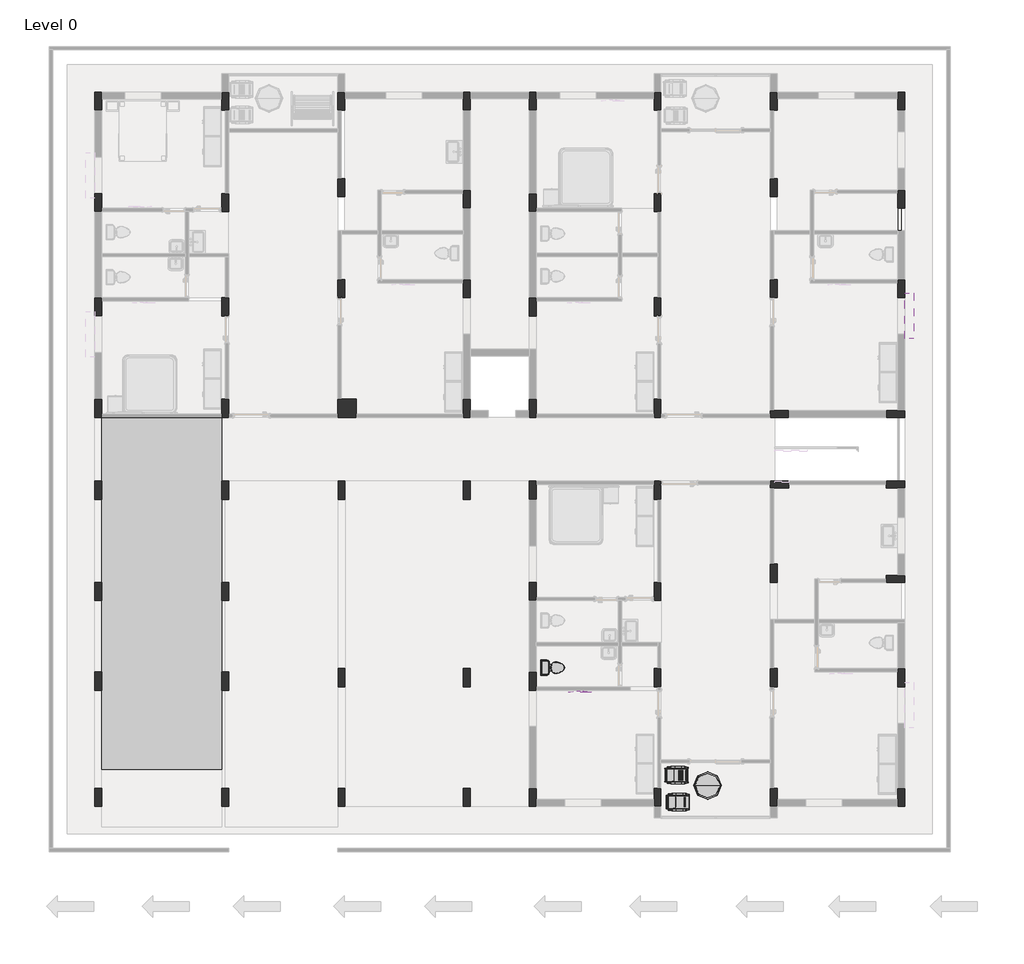
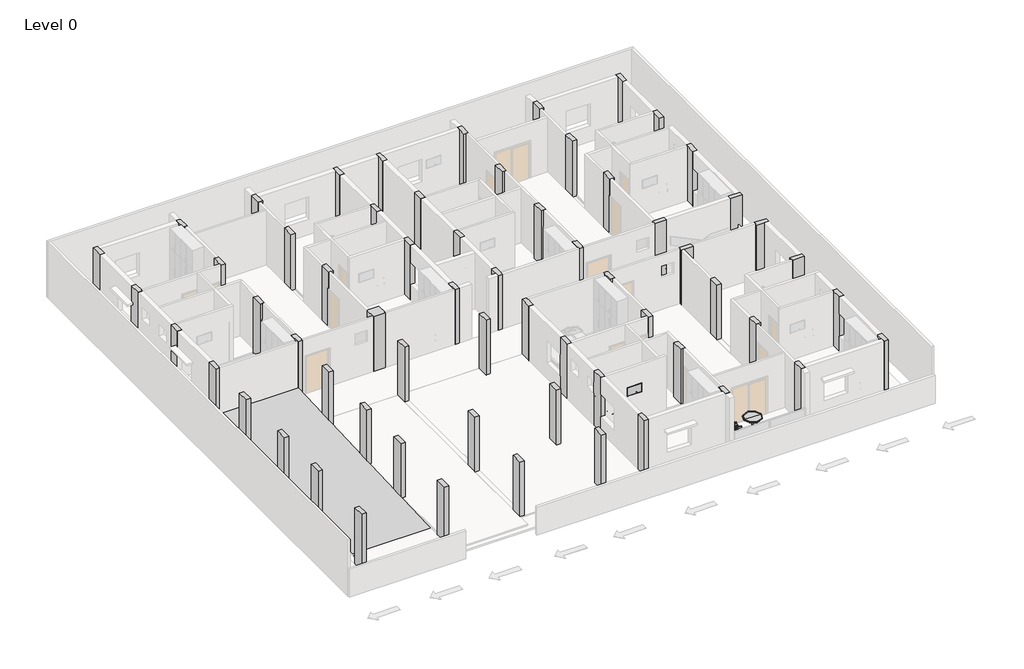
# One storey, part 5 of 6: 62 columns, 3 furniture elements, 2 slabs, 1 flow terminal, 1 proxy, 1 ramp.
"""IFC4 building model written with IfcOpenShell, lengths in millimetres."""

from ifc_helpers import new_model, si_unit, frame, origin, origin_with_axes, place, context, project, spatial, polyline, outline, extrude, faceted_brep, transform, mapped, element, save
from components import proxy_caca515e, concrete_rectangular_column_147977c2, concrete_rectangular_column_c091e905, toilet_domestic_3d_toilet_domestic_3d_ba6479b0, toilet_domestic_3d_toilet_domestic_3d_30431060, furniture_f9efd34a, adjustable_garden_chair_5339_adjustable_garden_chair_5339_e938936b, adjustable_garden_chair_5339_adjustable_garden_chair_5339_fbaf4b35, standard_832cbf63

model = new_model("IFC4")

# Units and contexts
model_context = context("Model", 3, world=origin())
ifc_project = project(units=[si_unit("LENGTHUNIT", "METRE", prefix="MILLI")], contexts=[model_context])

# Site, building, storey
site = spatial("IfcSite", under=ifc_project)
building = spatial("IfcBuilding", under=site)
storey = spatial("IfcBuildingStorey", under=building, Name="Level 0", Elevation=0.0)

# Proxy
placement = place(None, origin())
proxy_shape = proxy_caca515e(model_context)
element("IfcBuildingElementProxy", 1, Name="32\" ES6305U", ObjectType="32\" ES6305U", at=placement, inside=storey, context=model_context, shape_type="MappedRepresentation", body=[
    mapped(proxy_shape, transform((2883.4858266, -9593.9017861, 0.0), x_axis=(-1.0, 0.0, 0.0), y_axis=(0.0, -1.0, 0.0), z_axis=(0.0, 0.0, 1.0))),
])

# Columns
element("IfcColumn", 2, ObjectType="Concrete-Rectangular-Column", at=placement, inside=storey, context=model_context, shape_type="Brep", body=[
    faceted_brep([(-13249.7901539, 10361.8562752, 0.0), (-13249.7901539, 10133.2562752, 0.0), (-13249.7901539, 9752.2562752, 0.0), (-13478.3901539, 9752.2562752, 0.0), (-13478.3901539, 10361.8562752, 0.0), (-13249.7901539, 10361.8562752, 3048.0), (-13249.7901539, 10133.2562752, 3048.0), (-13249.7901539, 9752.2562752, 3048.0), (-13478.3901539, 9752.2562752, 3048.0), (-13478.3901539, 10361.8562752, 3048.0)], [[[0, 1, 2, 3, 4]], [[5, 6, 7, 2, 1, 0]], [[7, 8, 3, 2]], [[8, 9, 4, 3]], [[9, 5, 0, 4]], [[5, 9, 8, 7, 6]]]),
])
element("IfcColumn", 3, ObjectType="Concrete-Rectangular-Column", at=placement, inside=storey, context=model_context, shape_type="Brep", body=[
    faceted_brep([(-13249.7901539, 6972.1022446, 0.0), (-13249.7901539, 6362.5022446, 0.0), (-13478.3901539, 6362.5022446, 0.0), (-13478.3901539, 6972.1022446, 0.0), (-13249.7901539, 6972.1022446, 3048.0), (-13249.7901539, 6362.5022446, 3048.0), (-13249.7901539, 6972.1022446, 914.4), (-13249.7901539, 6972.1022446, 2133.6), (-13478.3901539, 6362.5022446, 3048.0), (-13478.3901539, 6972.1022446, 3048.0), (-13478.3901539, 6972.1022446, 2133.6), (-13478.3901539, 6972.1022446, 914.4)], [[[0, 1, 2, 3]], [[4, 5, 1, 0, 6, 7]], [[5, 8, 2, 1]], [[8, 9, 10, 11, 3, 2]], [[9, 4, 7, 6, 0, 3, 11, 10]], [[4, 9, 8, 5]]]),
])
element("IfcColumn", 4, ObjectType="Concrete-Rectangular-Column", at=placement, inside=storey, context=model_context, shape_type="SweptSolid", body=[
    extrude(outline(polyline([(-13249.7901539, 89.8788513), (-13249.7901539, -519.7211487), (-13478.3901539, -519.7211487), (-13478.3901539, 89.8788513), (-13249.7901539, 89.8788513)])), origin_with_axes(), (0.0, 0.0, 1.0), 3048.0),
])
element("IfcColumn", 5, ObjectType="Concrete-Rectangular-Column", at=placement, inside=storey, context=model_context, shape_type="Brep", body=[
    faceted_brep([(-9001.6401539, 10361.8562752, 0.0), (-9001.6401539, 9752.2562752, 0.0), (-9230.2401539, 9752.2562752, 0.0), (-9230.2401539, 10133.2562752, 0.0), (-9230.2401539, 10361.8562752, 0.0), (-9229.64062, 10361.8562752, 0.0), (-9001.6401539, 10361.8562752, 3048.0), (-9001.6401539, 9752.2562752, 3048.0), (-9230.2401539, 9752.2562752, 3048.0), (-9230.2401539, 10133.2562752, 3048.0), (-9230.2401539, 10361.8562752, 3048.0), (-9229.64062, 10361.8562752, 3048.0)], [[[0, 1, 2, 3, 4, 5]], [[6, 7, 1, 0]], [[7, 8, 2, 1]], [[8, 9, 10, 4, 3, 2]], [[10, 11, 6, 0, 5, 4]], [[6, 11, 10, 9, 8, 7]]]),
])
element("IfcColumn", 6, ObjectType="Concrete-Rectangular-Column", at=placement, inside=storey, context=model_context, shape_type="Brep", body=[
    faceted_brep([(-5115.4401539, 10364.1482139, 0.0), (-5115.4401539, 10363.0022446, 0.0), (-5115.4401539, 10134.4022446, 0.0), (-5115.4401539, 9754.5482139, 0.0), (-5344.0401539, 9754.5482139, 0.0), (-5344.0401539, 10364.1482139, 0.0), (-5115.4401539, 10364.1482139, 3048.0), (-5115.4401539, 10363.0022446, 3048.0), (-5115.4401539, 10134.4022446, 3048.0), (-5115.4401539, 9754.5482139, 3048.0), (-5344.0401539, 9754.5482139, 3048.0), (-5344.0401539, 10364.1482139, 3048.0)], [[[0, 1, 2, 3, 4, 5]], [[6, 7, 8, 9, 3, 2, 1, 0]], [[9, 10, 4, 3]], [[10, 11, 5, 4]], [[11, 6, 0, 5]], [[6, 11, 10, 9, 8, 7]]]),
])
element("IfcColumn", 7, ObjectType="Concrete-Rectangular-Column", at=placement, inside=storey, context=model_context, shape_type="Brep", body=[
    faceted_brep([(-924.4401539, 10363.0022446, 0.0), (-924.4401539, 10134.4022446, 0.0), (-924.4401539, 9753.4022446, 0.0), (-1153.0401539, 9753.4022446, 0.0), (-1153.0401539, 10134.4022446, 0.0), (-1153.0401539, 10363.0022446, 0.0), (-924.4401539, 10363.0022446, 3048.0), (-924.4401539, 10134.4022446, 3048.0), (-924.4401539, 9753.4022446, 3048.0), (-1153.0401539, 9753.4022446, 3048.0), (-1153.0401539, 10134.4022446, 3048.0), (-1153.0401539, 10363.0022446, 3048.0)], [[[0, 1, 2, 3, 4, 5]], [[6, 7, 8, 2, 1, 0]], [[8, 9, 3, 2]], [[9, 10, 11, 5, 4, 3]], [[11, 6, 0, 5]], [[6, 11, 10, 9, 8, 7]]]),
])
element("IfcColumn", 8, ObjectType="Concrete-Rectangular-Column", at=placement, inside=storey, context=model_context, shape_type="Brep", body=[
    faceted_brep([(1285.3598461, 10363.0022446, 0.0), (1285.3598461, 10134.4022446, 0.0), (1285.3598461, 9753.4022446, 0.0), (1056.7598461, 9753.4022446, 0.0), (1056.7598461, 10134.4022446, 0.0), (1056.7598461, 10363.0022446, 0.0), (1285.3598461, 10363.0022446, 3048.0), (1285.3598461, 10134.4022446, 3048.0), (1285.3598461, 9753.4022446, 3048.0), (1056.7598461, 9753.4022446, 3048.0), (1056.7598461, 10134.4022446, 3048.0), (1056.7598461, 10363.0022446, 3048.0)], [[[0, 1, 2, 3, 4, 5]], [[6, 7, 8, 2, 1, 0]], [[8, 9, 3, 2]], [[9, 10, 11, 5, 4, 3]], [[11, 6, 0, 5]], [[6, 11, 10, 9, 8, 7]]]),
])
element("IfcColumn", 9, ObjectType="Concrete-Rectangular-Column", at=placement, inside=storey, context=model_context, shape_type="Brep", body=[
    faceted_brep([(5457.3098461, 10364.1482139, 0.0), (5457.3098461, 9754.5482139, 0.0), (5228.7098461, 9754.5482139, 0.0), (5228.7098461, 10134.4022446, 0.0), (5228.7098461, 10363.0022446, 0.0), (5228.7098461, 10364.1482139, 0.0), (5457.3098461, 10364.1482139, 3048.0), (5457.3098461, 9754.5482139, 3048.0), (5228.7098461, 9754.5482139, 3048.0), (5228.7098461, 10134.4022446, 3048.0), (5228.7098461, 10363.0022446, 3048.0), (5228.7098461, 10364.1482139, 3048.0)], [[[0, 1, 2, 3, 4, 5]], [[6, 7, 1, 0]], [[7, 8, 2, 1]], [[8, 9, 10, 11, 5, 4, 3, 2]], [[11, 6, 0, 5]], [[6, 11, 10, 9, 8, 7]]]),
])
element("IfcColumn", 10, ObjectType="Concrete-Rectangular-Column", at=placement, inside=storey, context=model_context, shape_type="Brep", body=[
    faceted_brep([(9343.5098461, 10364.1482139, 0.0), (9343.5098461, 10135.5482139, 0.0), (9343.5098461, 9754.5482139, 0.0), (9114.9098461, 9754.5482139, 0.0), (9114.9098461, 10364.1482139, 0.0), (9343.5098461, 10364.1482139, 3048.0), (9343.5098461, 10135.5482139, 3048.0), (9343.5098461, 9754.5482139, 3048.0), (9114.9098461, 9754.5482139, 3048.0), (9114.9098461, 10364.1482139, 3048.0)], [[[0, 1, 2, 3, 4]], [[5, 6, 7, 2, 1, 0]], [[7, 8, 3, 2]], [[8, 9, 4, 3]], [[9, 5, 0, 4]], [[5, 9, 8, 7, 6]]]),
])
element("IfcColumn", 11, ObjectType="Concrete-Rectangular-Column", at=placement, inside=storey, context=model_context, shape_type="Brep", body=[
    faceted_brep([(13610.7098461, 10364.1482139, 0.0), (13610.7098461, 9754.5482139, 0.0), (13382.1098461, 9754.5482139, 0.0), (13382.1098461, 10135.5482139, 0.0), (13382.1098461, 10364.1482139, 0.0), (13610.7098461, 10364.1482139, 3048.0), (13610.7098461, 9754.5482139, 3048.0), (13382.1098461, 9754.5482139, 3048.0), (13382.1098461, 10135.5482139, 3048.0), (13382.1098461, 10364.1482139, 3048.0)], [[[0, 1, 2, 3, 4]], [[5, 6, 1, 0]], [[6, 7, 2, 1]], [[7, 8, 9, 4, 3, 2]], [[9, 5, 0, 4]], [[5, 9, 8, 7, 6]]]),
])
element("IfcColumn", 12, ObjectType="Concrete-Rectangular-Column", at=placement, inside=storey, context=model_context, shape_type="SweptSolid", body=[
    extrude(outline(polyline([(13610.7098461, 7086.4022446), (13610.7098461, 6476.8022446), (13382.1098461, 6476.8022446), (13382.1098461, 7086.4022446), (13610.7098461, 7086.4022446)])), origin_with_axes(), (0.0, 0.0, 1.0), 3048.0),
])
element("IfcColumn", 13, ObjectType="Concrete-Rectangular-Column", at=placement, inside=storey, context=model_context, shape_type="SweptSolid", body=[
    extrude(outline(polyline([(13610.7098465, 4090.3482139), (13610.7098465, 3480.7482139), (13382.1098465, 3480.7482139), (13382.1098465, 4090.3482139), (13610.7098465, 4090.3482139)])), origin_with_axes(), (0.0, 0.0, 1.0), 3048.0),
])
element("IfcColumn", 14, ObjectType="Concrete-Rectangular-Column", at=placement, inside=storey, context=model_context, shape_type="Brep", body=[
    faceted_brep([(13001.1098461, -291.1492785, 0.0), (13382.1098461, -291.1492785, 0.0), (13610.7098461, -291.1492785, 0.0), (13610.7098461, -519.7492785, 0.0), (13001.1098461, -519.7492785, 0.0), (13001.1098461, -291.1492785, 3048.0), (13382.1098461, -291.1492785, 3048.0), (13610.7098461, -291.1492785, 3048.0), (13610.7098461, -519.7492785, 3048.0), (13001.1098461, -519.7492785, 3048.0)], [[[0, 1, 2, 3, 4]], [[5, 6, 7, 2, 1, 0]], [[7, 8, 3, 2]], [[8, 9, 4, 3]], [[9, 5, 0, 4]], [[5, 9, 8, 7, 6]]]),
])
element("IfcColumn", 15, ObjectType="Concrete-Rectangular-Column", at=placement, inside=storey, context=model_context, shape_type="SweptSolid", body=[
    extrude(outline(polyline([(9116.1585903, -291.1517861), (9725.7585903, -291.1517861), (9725.7585903, -519.7517861), (9116.1585903, -519.7517861), (9116.1585903, -291.1517861)])), origin_with_axes(), (0.0, 0.0, 1.0), 3048.0),
])
element("IfcColumn", 16, ObjectType="Concrete-Rectangular-Column", at=placement, inside=storey, context=model_context, shape_type="Brep", body=[
    faceted_brep([(1056.7598461, -519.6614995, 0.0), (1056.7598461, -291.1517862, 0.0), (1056.7598461, 89.9385005, 0.0), (1285.3598461, 89.9385005, 0.0), (1285.3598461, -519.6614995, 0.0), (1056.7598461, -519.6614995, 3048.0), (1056.7598461, -291.1517862, 3048.0), (1056.7598461, 89.9385005, 3048.0), (1285.3598461, 89.9385005, 3048.0), (1285.3598461, -519.6614995, 3048.0)], [[[0, 1, 2, 3, 4]], [[5, 6, 7, 2, 1, 0]], [[7, 8, 3, 2]], [[8, 9, 4, 3]], [[9, 5, 0, 4]], [[5, 9, 8, 7, 6]]]),
])
element("IfcColumn", 17, ObjectType="Concrete-Rectangular-Column", at=placement, inside=storey, context=model_context, shape_type="Brep", body=[
    faceted_brep([(-1153.0401539, -519.7517861, 0.0), (-1153.0401539, 89.8482139, 0.0), (-924.4401539, 89.8482139, 0.0), (-924.4401539, -291.1517861, 0.0), (-924.4401539, -519.7517861, 0.0), (-1153.0401539, -519.7517861, 3048.0), (-1153.0401539, 89.8482139, 3048.0), (-924.4401539, 89.8482139, 3048.0), (-924.4401539, -291.1517861, 3048.0), (-924.4401539, -519.7517861, 3048.0)], [[[0, 1, 2, 3, 4]], [[5, 6, 1, 0]], [[6, 7, 2, 1]], [[7, 8, 9, 4, 3, 2]], [[9, 5, 0, 4]], [[5, 9, 8, 7, 6]]]),
])
element("IfcColumn", 18, ObjectType="Concrete-Rectangular-Column", at=placement, inside=storey, context=model_context, shape_type="SweptSolid", body=[
    extrude(outline(polyline([(1056.7598461, -3262.9517861), (1056.7598461, -2653.3517861), (1285.3598461, -2653.3517861), (1285.3598461, -3262.9517861), (1056.7598461, -3262.9517861)])), origin_with_axes(), (0.0, 0.0, 1.0), 3048.0),
])
element("IfcColumn", 19, ObjectType="Concrete-Rectangular-Column", at=placement, inside=storey, context=model_context, shape_type="Brep", body=[
    faceted_brep([(13610.7098461, -2881.9517861, 0.0), (13382.1098461, -2881.9517861, 0.0), (13001.1098461, -2881.9517861, 0.0), (13001.1098461, -2653.3517861, 0.0), (13610.7098461, -2653.3517861, 0.0), (13610.7098461, -2881.9517861, 3048.0), (13382.1098461, -2881.9517861, 3048.0), (13001.1098461, -2881.9517861, 3048.0), (13001.1098461, -2653.3517861, 3048.0), (13610.7098461, -2653.3517861, 3048.0)], [[[0, 1, 2, 3, 4]], [[5, 6, 7, 2, 1, 0]], [[7, 8, 3, 2]], [[8, 9, 4, 3]], [[9, 5, 0, 4]], [[5, 9, 8, 7, 6]]]),
])
element("IfcColumn", 20, ObjectType="Concrete-Rectangular-Column", at=placement, inside=storey, context=model_context, shape_type="Brep", body=[
    faceted_brep([(13610.7098461, -6044.2517861, 0.0), (13001.1098461, -6044.2517861, 0.0), (13001.1098461, -5815.6517861, 0.0), (13382.1098461, -5815.6517861, 0.0), (13610.7098461, -5815.6517861, 0.0), (13610.7098461, -6044.2517861, 3048.0), (13001.1098461, -6044.2517861, 3048.0), (13001.1098461, -5815.6517861, 3048.0), (13382.1098461, -5815.6517861, 3048.0), (13610.7098461, -5815.6517861, 3048.0)], [[[0, 1, 2, 3, 4]], [[5, 6, 1, 0]], [[6, 7, 2, 1]], [[7, 8, 9, 4, 3, 2]], [[9, 5, 0, 4]], [[5, 9, 8, 7, 6]]]),
])
element("IfcColumn", 21, ObjectType="Concrete-Rectangular-Column", at=placement, inside=storey, context=model_context, shape_type="Brep", body=[
    faceted_brep([(1285.3598461, -6044.2517861, 0.0), (1285.3598461, -6653.8517861, 0.0), (1056.7598461, -6653.8517861, 0.0), (1056.7598461, -6044.2517861, 0.0), (1285.3598461, -6044.2517861, 3048.0), (1285.3598461, -6653.8517861, 3048.0), (1285.3598461, -6044.2517861, 914.4), (1285.3598461, -6044.2517861, 2133.6), (1056.7598461, -6653.8517861, 3048.0), (1056.7598461, -6044.2517861, 3048.0), (1056.7598461, -6044.2517861, 2133.6), (1056.7598461, -6044.2517861, 914.4)], [[[0, 1, 2, 3]], [[4, 5, 1, 0, 6, 7]], [[5, 8, 2, 1]], [[8, 9, 10, 11, 3, 2]], [[9, 4, 7, 6, 0, 3, 11, 10]], [[4, 9, 8, 5]]]),
])
element("IfcColumn", 22, ObjectType="Concrete-Rectangular-Column", at=placement, inside=storey, context=model_context, shape_type="Brep", body=[
    faceted_brep([(1285.3598461, -12927.6517861, 0.0), (1285.3598461, -13308.6517861, 0.0), (1285.3598461, -13537.2517861, 0.0), (1056.7598461, -13537.2517861, 0.0), (1056.7598461, -12927.6517861, 0.0), (1285.3598461, -12927.6517861, 3048.0), (1285.3598461, -13308.6517861, 3048.0), (1285.3598461, -13537.2517861, 3048.0), (1056.7598461, -13537.2517861, 3048.0), (1056.7598461, -12927.6517861, 3048.0)], [[[0, 1, 2, 3, 4]], [[5, 6, 7, 2, 1, 0]], [[7, 8, 3, 2]], [[8, 9, 4, 3]], [[9, 5, 0, 4]], [[5, 9, 8, 7, 6]]]),
])
element("IfcColumn", 23, ObjectType="Concrete-Rectangular-Column", at=placement, inside=storey, context=model_context, shape_type="Brep", body=[
    faceted_brep([(5457.90938, -12927.6517861, 0.0), (5457.90938, -13537.2517861, 0.0), (5229.30938, -13537.2517861, 0.0), (5229.30938, -13308.6517861, 0.0), (5229.30938, -12927.6517861, 0.0), (5457.90938, -12927.6517861, 3048.0), (5457.90938, -13537.2517861, 3048.0), (5229.30938, -13537.2517861, 3048.0), (5229.30938, -13308.6517861, 3048.0), (5229.30938, -12927.6517861, 3048.0)], [[[0, 1, 2, 3, 4]], [[5, 6, 1, 0]], [[6, 7, 2, 1]], [[7, 8, 9, 4, 3, 2]], [[9, 5, 0, 4]], [[5, 9, 8, 7, 6]]]),
])
element("IfcColumn", 24, ObjectType="Concrete-Rectangular-Column", at=placement, inside=storey, context=model_context, shape_type="Brep", body=[
    faceted_brep([(9343.5098461, -12927.6517861, 0.0), (9343.5098461, -13308.6517861, 0.0), (9343.5098461, -13537.2517861, 0.0), (9114.9098461, -13537.2517861, 0.0), (9114.9098461, -12927.6517861, 0.0), (9343.5098461, -12927.6517861, 3048.0), (9343.5098461, -13308.6517861, 3048.0), (9343.5098461, -13537.2517861, 3048.0), (9114.9098461, -13537.2517861, 3048.0), (9114.9098461, -12927.6517861, 3048.0)], [[[0, 1, 2, 3, 4]], [[5, 6, 7, 2, 1, 0]], [[7, 8, 3, 2]], [[8, 9, 4, 3]], [[9, 5, 0, 4]], [[5, 9, 8, 7, 6]]]),
])
element("IfcColumn", 25, ObjectType="Concrete-Rectangular-Column", at=placement, inside=storey, context=model_context, shape_type="Brep", body=[
    faceted_brep([(13610.7098461, -12927.6517861, 0.0), (13610.7098461, -13537.2517861, 0.0), (13382.1098461, -13537.2517861, 0.0), (13382.1098461, -13308.6517861, 0.0), (13382.1098461, -12927.6517861, 0.0), (13610.7098461, -12927.6517861, 3048.0), (13610.7098461, -13537.2517861, 3048.0), (13382.1098461, -13537.2517861, 3048.0), (13382.1098461, -13308.6517861, 3048.0), (13382.1098461, -12927.6517861, 3048.0)], [[[0, 1, 2, 3, 4]], [[5, 6, 1, 0]], [[6, 7, 2, 1]], [[7, 8, 9, 4, 3, 2]], [[9, 5, 0, 4]], [[5, 9, 8, 7, 6]]]),
])
element("IfcColumn", 26, ObjectType="Concrete-Rectangular-Column", at=placement, inside=storey, context=model_context, shape_type="Brep", body=[
    faceted_brep([(13610.7098461, -8927.1824236, 0.0), (13610.7098461, -9536.7824236, 0.0), (13382.1098461, -9536.7824236, 0.0), (13382.1098461, -8927.1824236, 0.0), (13610.7098461, -8927.1824236, 3048.0), (13610.7098461, -9536.7824236, 3048.0), (13610.7098461, -9536.7824236, 2133.6), (13610.7098461, -9536.7824236, 914.4), (13382.1098461, -9536.7824236, 3048.0), (13382.1098461, -9536.7824236, 2133.6), (13382.1098461, -9536.7824236, 914.4), (13382.1098461, -8927.1824236, 3048.0)], [[[0, 1, 2, 3]], [[4, 5, 6, 7, 1, 0]], [[5, 8, 9, 10, 2, 1, 7, 6]], [[8, 11, 3, 2, 10, 9]], [[11, 4, 0, 3]], [[4, 11, 8, 5]]]),
])
element("IfcColumn", 27, ObjectType="Concrete-Rectangular-Column", at=placement, inside=storey, context=model_context, shape_type="Brep", body=[
    faceted_brep([(1285.3598461, -9041.4517861, 0.0), (1285.3598461, -9651.0517861, 0.0), (1056.7598461, -9651.0517861, 0.0), (1056.7598461, -9041.4517861, 0.0), (1285.3598461, -9041.4517861, 3048.0), (1285.3598461, -9651.0517861, 3048.0), (1285.3598461, -9651.0517861, 2133.6), (1285.3598461, -9651.0517861, 914.4), (1285.3598461, -9041.4517861, 1828.8), (1285.3598461, -9041.4517861, 2438.4), (1056.7598461, -9651.0517861, 3048.0), (1056.7598461, -9651.0517861, 2133.6), (1056.7598461, -9651.0517861, 914.4), (1056.7598461, -9041.4517861, 3048.0), (1056.7598461, -9041.4517861, 2438.4), (1056.7598461, -9041.4517861, 1828.8)], [[[0, 1, 2, 3]], [[4, 5, 6, 7, 1, 0, 8, 9]], [[5, 10, 11, 12, 2, 1, 7, 6]], [[10, 13, 14, 15, 3, 2, 12, 11]], [[13, 4, 9, 8, 0, 3, 15, 14]], [[4, 13, 10, 5]]]),
])
element("IfcColumn", 28, ObjectType="Concrete-Rectangular-Column", at=placement, inside=storey, context=model_context, shape_type="Brep", body=[
    faceted_brep([(-924.4401539, 4089.2022446, 0.0), (-924.4401539, 3479.6022446, 0.0), (-1153.0401539, 3479.6022446, 0.0), (-1153.0401539, 4089.2022446, 0.0), (-924.4401539, 4089.2022446, 3048.0), (-924.4401539, 3479.6022446, 3048.0), (-924.4401539, 3479.6022446, 2133.6), (-924.4401539, 3479.6022446, 914.4), (-1153.0401539, 3479.6022446, 3048.0), (-1153.0401539, 3479.6022446, 2133.6), (-1153.0401539, 3479.6022446, 914.4), (-1153.0401539, 4089.2022446, 3048.0)], [[[0, 1, 2, 3]], [[4, 5, 6, 7, 1, 0]], [[5, 8, 9, 10, 2, 1, 7, 6]], [[8, 11, 3, 2, 10, 9]], [[11, 4, 0, 3]], [[4, 11, 8, 5]]]),
])
element("IfcColumn", 29, ObjectType="Concrete-Rectangular-Column", at=placement, inside=storey, context=model_context, shape_type="Brep", body=[
    faceted_brep([(1285.3598461, 3481.8941832, 0.0), (1285.3598461, 2872.2941832, 0.0), (1056.7598461, 2872.2941832, 0.0), (1056.7598461, 3481.8941832, 0.0), (1285.3598461, 3481.8941832, 3048.0), (1285.3598461, 2872.2941832, 3048.0), (1285.3598461, 2872.2941832, 2133.6), (1285.3598461, 2872.2941832, 914.4), (1056.7598461, 2872.2941832, 3048.0), (1056.7598461, 2872.2941832, 2133.6), (1056.7598461, 2872.2941832, 914.4), (1056.7598461, 3481.8941832, 3048.0)], [[[0, 1, 2, 3]], [[4, 5, 6, 7, 1, 0]], [[5, 8, 9, 10, 2, 1, 7, 6]], [[8, 11, 3, 2, 10, 9]], [[11, 4, 0, 3]], [[4, 11, 8, 5]]]),
])
element("IfcColumn", 30, ObjectType="Concrete-Rectangular-Column", at=placement, inside=storey, context=model_context, shape_type="Brep", body=[
    faceted_brep([(1285.3598461, 6972.1022446, 0.0), (1285.3598461, 6477.9482139, 0.0), (1285.3598461, 6363.6482139, 0.0), (1285.3598461, 6362.5022446, 0.0), (1056.7598461, 6362.5022446, 0.0), (1056.7598461, 6972.1022446, 0.0), (1285.3598461, 6972.1022446, 3048.0), (1285.3598461, 6477.9482139, 3048.0), (1285.3598461, 6363.6482139, 3048.0), (1285.3598461, 6362.5022446, 3048.0), (1056.7598461, 6362.5022446, 3048.0), (1056.7598461, 6972.1022446, 3048.0)], [[[0, 1, 2, 3, 4, 5]], [[6, 7, 8, 9, 3, 2, 1, 0]], [[9, 10, 4, 3]], [[10, 11, 5, 4]], [[11, 6, 0, 5]], [[6, 11, 10, 9, 8, 7]]]),
])
element("IfcColumn", 31, ObjectType="Concrete-Rectangular-Column", at=placement, inside=storey, context=model_context, shape_type="SweptSolid", body=[
    extrude(outline(polyline([(-924.4401539, 7087.5482139), (-924.4401539, 6477.9482139), (-1153.0401539, 6477.9482139), (-1153.0401539, 7087.5482139), (-924.4401539, 7087.5482139)])), origin_with_axes(), (0.0, 0.0, 1.0), 3048.0),
])
element("IfcColumn", 32, ObjectType="Concrete-Rectangular-Column", at=placement, inside=storey, context=model_context, shape_type="SweptSolid", body=[
    extrude(outline(polyline([(-13249.7901539, 3480.7482139), (-13249.7901539, 2871.1482139), (-13478.3901539, 2871.1482139), (-13478.3901539, 3480.7482139), (-13249.7901539, 3480.7482139)])), origin_with_axes(), (0.0, 0.0, 1.0), 3048.0),
])
concrete_rectangular_column_shape = concrete_rectangular_column_147977c2(model_context)
element("IfcColumn", 33, ObjectType="Concrete-Rectangular-Column", at=placement, inside=storey, context=model_context, shape_type="MappedRepresentation", body=[
    mapped(concrete_rectangular_column_shape, transform((-9115.9401539, -214.9211487, 0.0), x_axis=(1.0, 0.0, 0.0), y_axis=(0.0, 1.0, 0.0), z_axis=(0.0, 0.0, 1.0))),
])
element("IfcColumn", 34, ObjectType="Concrete-Rectangular-Column", at=placement, inside=storey, context=model_context, shape_type="MappedRepresentation", body=[
    mapped(concrete_rectangular_column_shape, transform((5343.0098461, -214.8614995, 0.0), x_axis=(-1.0, 0.0, 0.0), y_axis=(0.0, -1.0, 0.0), z_axis=(0.0, 0.0, 1.0))),
])
element("IfcColumn", 35, ObjectType="Concrete-Rectangular-Column", at=placement, inside=storey, context=model_context, shape_type="MappedRepresentation", body=[
    mapped(concrete_rectangular_column_shape, transform((-5228.2486431, -2957.0057655, 0.0), x_axis=(-1.0, 0.0, 0.0), y_axis=(0.0, -1.0, 0.0), z_axis=(0.0, 0.0, 1.0))),
])
element("IfcColumn", 36, ObjectType="Concrete-Rectangular-Column", at=placement, inside=storey, context=model_context, shape_type="MappedRepresentation", body=[
    mapped(concrete_rectangular_column_shape, transform((-9115.9401539, -2958.1517861, 0.0), x_axis=(-1.0, 0.0, 0.0), y_axis=(0.0, -1.0, 0.0), z_axis=(0.0, 0.0, 1.0))),
])
element("IfcColumn", 37, ObjectType="Concrete-Rectangular-Column", at=placement, inside=storey, context=model_context, shape_type="MappedRepresentation", body=[
    mapped(concrete_rectangular_column_shape, transform((-1037.927239, -2957.0057654, 0.0), x_axis=(-1.0, 0.0, 0.0), y_axis=(0.0, -1.0, 0.0), z_axis=(0.0, 0.0, 1.0))),
])
element("IfcColumn", 38, ObjectType="Concrete-Rectangular-Column", at=placement, inside=storey, context=model_context, shape_type="MappedRepresentation", body=[
    mapped(concrete_rectangular_column_shape, transform((5343.0096341, -2958.1517861, 0.0), x_axis=(-1.0, 0.0, 0.0), y_axis=(0.0, -1.0, 0.0), z_axis=(0.0, 0.0, 1.0))),
])
element("IfcColumn", 39, ObjectType="Concrete-Rectangular-Column", at=placement, inside=storey, context=model_context, shape_type="MappedRepresentation", body=[
    mapped(concrete_rectangular_column_shape, transform((9420.9585903, -2767.6517861, 0.0), x_axis=(0.0, -1.0, 0.0), y_axis=(1.0, 0.0, 0.0), z_axis=(0.0, 0.0, 1.0))),
])
element("IfcColumn", 40, ObjectType="Concrete-Rectangular-Column", at=placement, inside=storey, context=model_context, shape_type="MappedRepresentation", body=[
    mapped(concrete_rectangular_column_shape, transform((9229.2098461, -5739.4517861, 0.0), x_axis=(1.0, 0.0, 0.0), y_axis=(0.0, 1.0, 0.0), z_axis=(0.0, 0.0, 1.0))),
])
element("IfcColumn", 41, ObjectType="Concrete-Rectangular-Column", at=placement, inside=storey, context=model_context, shape_type="MappedRepresentation", body=[
    mapped(concrete_rectangular_column_shape, transform((5343.0098461, -6349.0517861, 0.0), x_axis=(1.0, 0.0, 0.0), y_axis=(0.0, 1.0, 0.0), z_axis=(0.0, 0.0, 1.0))),
])
element("IfcColumn", 42, ObjectType="Concrete-Rectangular-Column", at=placement, inside=storey, context=model_context, shape_type="MappedRepresentation", body=[
    mapped(concrete_rectangular_column_shape, transform((-1038.0863987, -9231.9517861, 0.0), x_axis=(1.0, 0.0, 0.0), y_axis=(0.0, 1.0, 0.0), z_axis=(0.0, 0.0, 1.0))),
])
element("IfcColumn", 43, ObjectType="Concrete-Rectangular-Column", at=placement, inside=storey, context=model_context, shape_type="MappedRepresentation", body=[
    mapped(concrete_rectangular_column_shape, transform((-5228.4078028, -9231.9517861, 0.0), x_axis=(1.0, 0.0, 0.0), y_axis=(0.0, 1.0, 0.0), z_axis=(0.0, 0.0, 1.0))),
])
element("IfcColumn", 44, ObjectType="Concrete-Rectangular-Column", at=placement, inside=storey, context=model_context, shape_type="MappedRepresentation", body=[
    mapped(concrete_rectangular_column_shape, transform((-5228.4078028, -13232.4517861, 0.0), x_axis=(1.0, 0.0, 0.0), y_axis=(0.0, 1.0, 0.0), z_axis=(0.0, 0.0, 1.0))),
])
element("IfcColumn", 45, ObjectType="Concrete-Rectangular-Column", at=placement, inside=storey, context=model_context, shape_type="MappedRepresentation", body=[
    mapped(concrete_rectangular_column_shape, transform((-1038.0863987, -13232.4517861, 0.0), x_axis=(1.0, 0.0, 0.0), y_axis=(0.0, 1.0, 0.0), z_axis=(0.0, 0.0, 1.0))),
])
element("IfcColumn", 46, ObjectType="Concrete-Rectangular-Column", at=placement, inside=storey, context=model_context, shape_type="MappedRepresentation", body=[
    mapped(concrete_rectangular_column_shape, transform((-9115.9401539, -13232.4517861, 0.0), x_axis=(1.0, 0.0, 0.0), y_axis=(0.0, 1.0, 0.0), z_axis=(0.0, 0.0, 1.0))),
])
element("IfcColumn", 47, ObjectType="Concrete-Rectangular-Column", at=placement, inside=storey, context=model_context, shape_type="MappedRepresentation", body=[
    mapped(concrete_rectangular_column_shape, transform((-9115.9401539, -9346.2517861, 0.0), x_axis=(1.0, 0.0, 0.0), y_axis=(0.0, 1.0, 0.0), z_axis=(0.0, 0.0, 1.0))),
])
element("IfcColumn", 48, ObjectType="Concrete-Rectangular-Column", at=placement, inside=storey, context=model_context, shape_type="MappedRepresentation", body=[
    mapped(concrete_rectangular_column_shape, transform((-9115.9401539, -6349.0517861, 0.0), x_axis=(1.0, 0.0, 0.0), y_axis=(0.0, 1.0, 0.0), z_axis=(0.0, 0.0, 1.0))),
])
element("IfcColumn", 49, ObjectType="Concrete-Rectangular-Column", at=placement, inside=storey, context=model_context, shape_type="MappedRepresentation", body=[
    mapped(concrete_rectangular_column_shape, transform((-13363.49062, -2958.1517861, 0.0), x_axis=(1.0, 0.0, 0.0), y_axis=(0.0, 1.0, 0.0), z_axis=(0.0, 0.0, 1.0))),
])
element("IfcColumn", 50, ObjectType="Concrete-Rectangular-Column", at=placement, inside=storey, context=model_context, shape_type="MappedRepresentation", body=[
    mapped(concrete_rectangular_column_shape, transform((-13364.0901539, -6349.0517861, 0.0), x_axis=(1.0, 0.0, 0.0), y_axis=(0.0, 1.0, 0.0), z_axis=(0.0, 0.0, 1.0))),
])
element("IfcColumn", 51, ObjectType="Concrete-Rectangular-Column", at=placement, inside=storey, context=model_context, shape_type="MappedRepresentation", body=[
    mapped(concrete_rectangular_column_shape, transform((-13364.0901539, -9346.2517861, 0.0), x_axis=(1.0, 0.0, 0.0), y_axis=(0.0, 1.0, 0.0), z_axis=(0.0, 0.0, 1.0))),
])
element("IfcColumn", 52, ObjectType="Concrete-Rectangular-Column", at=placement, inside=storey, context=model_context, shape_type="MappedRepresentation", body=[
    mapped(concrete_rectangular_column_shape, transform((-13364.0901539, -13232.4517861, 0.0), x_axis=(1.0, 0.0, 0.0), y_axis=(0.0, 1.0, 0.0), z_axis=(0.0, 0.0, 1.0))),
])
element("IfcColumn", 53, ObjectType="Concrete-Rectangular-Column", at=placement, inside=storey, context=model_context, shape_type="MappedRepresentation", body=[
    mapped(concrete_rectangular_column_shape, transform((9229.2098461, -9231.9517861, 0.0), x_axis=(1.0, 0.0, 0.0), y_axis=(0.0, 1.0, 0.0), z_axis=(0.0, 0.0, 1.0))),
])
element("IfcColumn", 54, ObjectType="Concrete-Rectangular-Column", at=placement, inside=storey, context=model_context, shape_type="MappedRepresentation", body=[
    mapped(concrete_rectangular_column_shape, transform((5343.0098461, -9231.9517861, 0.0), x_axis=(1.0, 0.0, 0.0), y_axis=(0.0, 1.0, 0.0), z_axis=(0.0, 0.0, 1.0))),
])
element("IfcColumn", 55, ObjectType="Concrete-Rectangular-Column", at=placement, inside=storey, context=model_context, shape_type="MappedRepresentation", body=[
    mapped(concrete_rectangular_column_shape, transform((-9115.9401539, 3177.0941832, 0.0), x_axis=(1.0, 0.0, 0.0), y_axis=(0.0, 1.0, 0.0), z_axis=(0.0, 0.0, 1.0))),
])
element("IfcColumn", 56, ObjectType="Concrete-Rectangular-Column", at=placement, inside=storey, context=model_context, shape_type="MappedRepresentation", body=[
    mapped(concrete_rectangular_column_shape, transform((-5229.7401539, 3785.5482139, 0.0), x_axis=(1.0, 0.0, 0.0), y_axis=(0.0, 1.0, 0.0), z_axis=(0.0, 0.0, 1.0))),
])
element("IfcColumn", 57, ObjectType="Concrete-Rectangular-Column", at=placement, inside=storey, context=model_context, shape_type="MappedRepresentation", body=[
    mapped(concrete_rectangular_column_shape, transform((5343.0098461, 3177.0941832, 0.0), x_axis=(1.0, 0.0, 0.0), y_axis=(0.0, 1.0, 0.0), z_axis=(0.0, 0.0, 1.0))),
])
element("IfcColumn", 58, ObjectType="Concrete-Rectangular-Column", at=placement, inside=storey, context=model_context, shape_type="MappedRepresentation", body=[
    mapped(concrete_rectangular_column_shape, transform((-5229.7401539, 7162.6022446, 0.0), x_axis=(1.0, 0.0, 0.0), y_axis=(0.0, 1.0, 0.0), z_axis=(0.0, 0.0, 1.0))),
])
element("IfcColumn", 59, ObjectType="Concrete-Rectangular-Column", at=placement, inside=storey, context=model_context, shape_type="MappedRepresentation", body=[
    mapped(concrete_rectangular_column_shape, transform((-9115.9401539, 6667.3022446, 0.0), x_axis=(1.0, 0.0, 0.0), y_axis=(0.0, 1.0, 0.0), z_axis=(0.0, 0.0, 1.0))),
])
element("IfcColumn", 60, ObjectType="Concrete-Rectangular-Column", at=placement, inside=storey, context=model_context, shape_type="MappedRepresentation", body=[
    mapped(concrete_rectangular_column_shape, transform((5343.0098461, 6667.3022446, 0.0), x_axis=(1.0, 0.0, 0.0), y_axis=(0.0, 1.0, 0.0), z_axis=(0.0, 0.0, 1.0))),
])
element("IfcColumn", 61, ObjectType="Concrete-Rectangular-Column", at=placement, inside=storey, context=model_context, shape_type="MappedRepresentation", body=[
    mapped(concrete_rectangular_column_shape, transform((9229.2098461, 3785.5482139, 0.0), x_axis=(1.0, 0.0, 0.0), y_axis=(0.0, 1.0, 0.0), z_axis=(0.0, 0.0, 1.0))),
])
element("IfcColumn", 62, ObjectType="Concrete-Rectangular-Column", at=placement, inside=storey, context=model_context, shape_type="MappedRepresentation", body=[
    mapped(concrete_rectangular_column_shape, transform((9232.3684396, 7163.7482139, 0.0), x_axis=(1.0, 0.0, 0.0), y_axis=(0.0, 1.0, 0.0), z_axis=(0.0, 0.0, 1.0))),
])
concrete_rectangular_column_2_shape = concrete_rectangular_column_c091e905(model_context)
element("IfcColumn", 63, ObjectType="Concrete-Rectangular-Column", at=placement, inside=storey, context=model_context, shape_type="MappedRepresentation", body=[
    mapped(concrete_rectangular_column_2_shape, transform((-5039.2401539, -214.9211487, 0.0), x_axis=(1.0, 0.0, 0.0), y_axis=(0.0, 1.0, 0.0), z_axis=(0.0, 0.0, 1.0))),
])

# Flow terminal
toilet_domestic_3d_toilet_domestic_3d_shape = toilet_domestic_3d_toilet_domestic_3d_ba6479b0(model_context)
toilet_domestic_3d_toilet_domestic_3d_2_shape = toilet_domestic_3d_toilet_domestic_3d_30431060(model_context)
element("IfcFlowTerminal", 64, ObjectType="Toilet-Domestic-3D : Toilet-Domestic-3D", at=placement, inside=storey, context=model_context, shape_type="MappedRepresentation", body=[
    mapped(toilet_domestic_3d_toilet_domestic_3d_shape, transform((1932.9236467, -8898.0865272, 0.0), x_axis=(0.0, 1.0, 0.0), y_axis=(-1.0, 0.0, 0.0), z_axis=(0.0, 0.0, 1.0))),
    mapped(toilet_domestic_3d_toilet_domestic_3d_2_shape, transform((1932.9236467, -8898.0865272, 0.0), x_axis=(0.0, 1.0, 0.0), y_axis=(-1.0, 0.0, 0.0), z_axis=(0.0, 0.0, 1.0))),
])

# Furniture
furniture_shape = furniture_f9efd34a(model_context)
element("IfcFurniture", 65, ObjectType="Table-Round : 36\" Diameter", at=placement, inside=storey, context=model_context, shape_type="MappedRepresentation", body=[
    mapped(furniture_shape, transform((7019.6258765, -12843.3118957, 0.0), x_axis=(1.0, 0.0, 0.0), y_axis=(0.0, 1.0, 0.0), z_axis=(0.0, 0.0, 1.0))),
])
adjustable_garden_chair_5339_adjustable_garden_chair_5339_shape = adjustable_garden_chair_5339_adjustable_garden_chair_5339_e938936b(model_context)
element("IfcFurniture", 66, ObjectType="adjustable_garden_chair_5339 : adjustable_garden_chair_5339", at=placement, inside=storey, context=model_context, shape_type="MappedRepresentation", body=[
    mapped(adjustable_garden_chair_5339_adjustable_garden_chair_5339_shape, transform((5967.8250218, -12495.8517861, 0.0), x_axis=(0.0, 1.0, 0.0), y_axis=(-1.0, 0.0, 0.0), z_axis=(0.0, 0.0, 1.0))),
])
adjustable_garden_chair_5339_adjustable_garden_chair_5339_2_shape = adjustable_garden_chair_5339_adjustable_garden_chair_5339_fbaf4b35(model_context)
element("IfcFurniture", 67, ObjectType="adjustable_garden_chair_5339 : adjustable_garden_chair_5339", at=placement, inside=storey, context=model_context, shape_type="MappedRepresentation", body=[
    mapped(adjustable_garden_chair_5339_adjustable_garden_chair_5339_2_shape, transform((6012.6715513, -13397.191043, 0.0), x_axis=(0.0, -1.0, 0.0), y_axis=(1.0, 0.0, 0.0), z_axis=(0.0, 0.0, 1.0))),
])

# Ramp
standard_shape = standard_832cbf63(model_context)
element("IfcRamp", 68, ObjectType="Standard", at=placement, inside=storey, context=model_context, shape_type="MappedRepresentation", body=[
    mapped(standard_shape, transform((0.0, 0.0, 0.0), x_axis=(1.0, 0.0, 0.0), y_axis=(0.0, 1.0, 0.0), z_axis=(0.0, 0.0, 1.0))),
])

# Slabs
element("IfcSlab", 69, at=placement, inside=storey, context=model_context, shape_type="Brep", body=[
    faceted_brep([(10562.6567877, 5727.5022446, -50.8), (10562.6567877, 6973.2482139, -50.8), (13382.1098461, 6973.2482139, -50.8), (13382.1098461, 6476.8022446, -50.8), (13496.4098461, 6476.8022446, -50.8), (13496.4098461, 5727.5022446, -50.8), (10562.6567877, 6973.2482139, 0.0), (10562.6567877, 5727.5022446, 0.0), (13496.4098461, 5727.5022446, 0.0), (13496.4098461, 6476.8022446, 0.0), (13382.1098461, 6476.8022446, 0.0), (13382.1098461, 6973.2482139, 0.0)], [[[0, 1, 2, 3, 4, 5]], [[6, 7, 8, 9, 10, 11]], [[1, 0, 7, 6]], [[2, 1, 6, 11]], [[3, 2, 11, 10]], [[4, 3, 10, 9]], [[5, 4, 9, 8]], [[0, 5, 8, 7]]]),
    faceted_brep([(9267.64644, -521.0312258, -50.8), (9267.64644, -2653.3517861, -50.8), (1056.7598461, -2653.3517861, -50.8), (-9001.6401539, -2653.3517861, -50.8), (-9115.9401539, -2653.3517861, -50.8), (-9115.9401539, -521.0312258, -50.8), (9267.64644, -2653.3517861, 0.0), (9267.64644, -521.0312258, 0.0), (-9115.9401539, -521.0312258, 0.0), (-9115.9401539, -2653.3517861, 0.0), (-9001.6401539, -2653.3517861, 0.0), (1056.7598461, -2653.3517861, 0.0)], [[[0, 1, 2, 3, 4, 5]], [[6, 7, 8, 9, 10, 11]], [[1, 0, 7, 6]], [[1, 6, 11, 10, 9, 4, 3, 2]], [[5, 4, 9, 8]], [[0, 5, 8, 7]]]),
])
element("IfcSlab", 70, ObjectType="4\"", at=placement, inside=storey, context=model_context, shape_type="SweptSolid", body=[
    extrude(outline(polyline([(13915.5098465, 2108.5870695), (13610.7098465, 2108.5870695), (13610.7098465, 3632.5870695), (13915.5098465, 3632.5870695), (13915.5098465, 2108.5870695)])), frame((0.0, 0.0, 2108.2), z_axis=(0.0, 0.0, 1.0), x_axis=(1.0, 0.0, 0.0)), (0.0, 0.0, 1.0), 101.6),
])

save(model, "model.ifc")

# Revit data of these elements
# Type "32\" ES6305U"
#   URL = "http://www.samsung.com"
#   Model = "32ES6305U"
#   Manufacturer = "Samsung"
#   Description = "3D led smart tv, 6 series"
#   Width = 2' - 5.13386"
#   Placement height [instance default] = 5' - 6.92913"
#   Outputs inset = 0' - 0.3937"
#   Output size = 0' - 0.15748"
#   Inset corners = 0' - 0.3937"
#   Inset component exit = 0' - 1.77165"
#   Inset body = 0' - 0.7874"
#   Height = 1' - 5.6378"
#   Depth screen = 0' - 0.62992"
#   Depth frame edge = 0' - 0.03937"
#   Depth distance = 0' - 1.1811"
#   Depth body = 0' - 0.86614"
#   Screen material = TV Screen material
#   Frame material = TV Frame material
#   Body material = TV Body material
#   Default Elevation = 0
# Type "Concrete-Rectangular-Column"
#   Assembly Code = "B10"
#   b = 0' - 9"
#   h = 2' - 0"
#   Structural Material [instance default] = Concrete, Cast-in-Place gray
# Type "Concrete-Rectangular-Column"
#   Assembly Code = "B10"
#   b = 2' - 0"
#   h = 2' - 0"
#   Structural Material [instance default] = Concrete, Cast-in-Place gray
# Type "Toilet-Domestic-3D : Toilet-Domestic-3D"
#   Assembly Code = "D2010110"
#   Toilet - Bowl/Basin Material = Porcelain, Linen
#   Toilet - Seat Material = Laminate, Linen, Matte
#   Default Elevation = 0
# Type "Table-Round : 36\" Diameter"
#   Assembly Code = "E2020200"
#   Base Radius = 0' - 10"
#   Height = 2' - 6"
#   Radius = 1' - 6"
#   Base Material = Steel, Chrome Plated
#   Top Material = Birch
#   Default Elevation = 0
# Type "adjustable_garden_chair_5339 : adjustable_garden_chair_5339"
#   URL = "www.revitlog.nl"
#   diepte = 2' - 7.49606"
#   corner back [instance default] = 120.00°
#   breedte = 1' - 8.07874"
#   kussen visible [instance default] = yes
#   stoel = hout
#   Default Elevation = 0
# Type "Standard"
#   built-in parameter 1008304 = 0.492126 (stored number, unit not read)
#   built-in parameter 1008303 = 12 (stored number, unit not read)
#   built-in parameter 1008301 = 25 (stored number, unit not read)
#   built-in parameter 1008305 = 1
#   Function = 1
# Type
#   Function = 0
#   Layers, outside or top first: 0' - 2" "Concrete" (function 1)
# Type "4\""
#   Function = 0
#   Layers, outside or top first: 0' - 4" "Concrete" (function 1)
# Element 1 (IfcBuildingElementProxy, "32\" ES6305U")
#   Placement height = 6' - 0"
#   Phase Created = New Construction
#   Materials on its faces: "TV Body material", "TV Frame material", "TV Screen material"
# Elements 2, 3, 4, 5, 6, 7, 8, 9, 10, 11, 12, 13, 14, 15, 16, 17, 18, 19, 20, 21, 22, 23, 24, 25, 26, 27, 28, 29, 30, 31, 32, 33, 34, 35, 36, 37, 38, 39, 40, 41, 42, 43, 44, 45, 46, 47, 48, 49, 50, 51, 52, 53, 54, 55, 56, 57, 58, 59, 60, 61, 62, 63 (IfcColumn, "Concrete-Rectangular-Column")
#   Structural Material = Concrete
#   Phase Created = New Construction
#   Materials on its faces: "Concrete"
# Element 64 (IfcFlowTerminal, "Toilet-Domestic-3D : Toilet-Domestic-3D")
#   Mark = "7"
#   Phase Created = New Construction
#   Materials on its faces: "Porcelain, Linen", "Laminate, Linen, Matte"
# Element 65 (IfcFurniture, "Table-Round : 36\" Diameter")
#   Phase Created = New Construction
#   Materials on its faces: "Steel, Chrome Plated", "Birch"
# Elements 66, 67 (IfcFurniture, "adjustable_garden_chair_5339 : adjustable_garden_chair_5339")
#   Phase Created = New Construction
#   Materials on its faces: "hout"
# Element 68 (IfcRamp, "Standard")
#   built-in parameter 1007275 = "DN"
#   built-in parameter 1007272 = "UP"
#   Width = 13' - 2"
#   built-in parameter 1007276 = 1
#   built-in parameter 1007274 = 1
#   built-in parameter 1007273 = 1
#   built-in parameter 1007271 = 1
#   Phase Created = New Construction
# Element 69 (IfcSlab)
#   built-in parameter 1001955 = 3.14159 (stored number, unit not read)
#   Height Offset From Level = 0' - 0"
#   Phase Created = New Construction
#   Materials on its faces: "Concrete"
# Element 70 (IfcSlab, "4\"")
#   built-in parameter 1001955 = -1.5708 (stored number, unit not read)
#   Height Offset From Level = 7' - 3"
#   Phase Created = New Construction
#   Materials on its faces: "Concrete"
# Materials
#   "TV Screen material": class "Plastic", colour RGB 5 5 5, transparency 0, Description = "Plastic, generic, opaque black", Cost = 0
#   "TV Frame material": class "Metal", colour RGB 244 244 244, transparency 0, Cost = 0
#   "TV Body material": class "Plastic", colour RGB 31 31 31, transparency 0, Description = "Plastic, generic, opaque dark grey", Cost = 0
#   "Concrete, Cast-in-Place gray": class "Concrete", colour RGB 192 192 192, transparency 0, Description = "Cast-in-place concrete", Cost = 0
#   "Porcelain, Linen": class "Ceramic", colour RGB 249 239 230, transparency 0, Description = "Porcelain, linen", Cost = 0
#   "Laminate, Linen, Matte": class "Plastic", colour RGB 249 239 230, transparency 0, Description = "Plastic Laminate - Linen, Matte", Cost = 0
#   "Steel, Chrome Plated": class "Metal", colour RGB 216 216 216, transparency 0, Description = "Chromiuim plated steel", Cost = 0
#   "Birch": class "Wood", colour RGB 224 178 126, transparency 0, Description = "Betula Alleghaniensis", Cost = 0
#   "hout": class "Wood", colour RGB 140 61 26, transparency 0
#   "Concrete": class "Concrete", colour RGB 120 120 120, transparency 0, Description = "Portland Cement Concrete", Cost = 0
